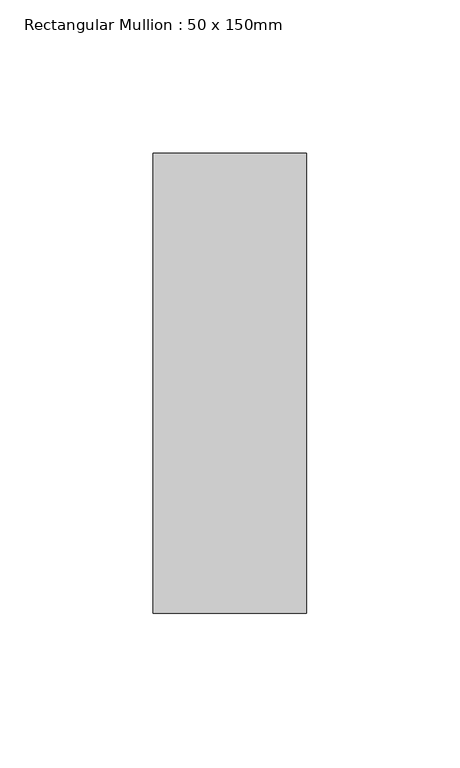
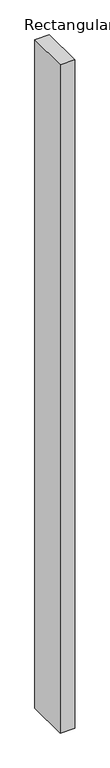
"""IFC4 building model written with IfcOpenShell, lengths in millimetres: member geometry, Rectangular Mullion : 50 x 150mm."""

from ifc_helpers import new_model, si_unit, frame, origin, place, context, project, spatial, polyline, outline, extrude, source, transform, mapped, element, save


def rectangular_mullion_50_x_150mm_fd5e96fe(model_context):
    return source(origin(), model_context, "Body", "SweptSolid", [
        extrude(outline(polyline([(0.0, 75.0), (0.0, -75.0), (-50.0, -75.0), (-50.0, 75.0), (0.0, 75.0)])), frame((0.0, 0.0, -2425.0), z_axis=(0.0, 0.0, 1.0), x_axis=(1.0, 0.0, 0.0)), (0.0, 0.0, 1.0), 2425.0),
    ])


if __name__ == "__main__":
    model = new_model("IFC4")
    model_context = context("Model", 3, world=origin())
    ifc_project = project(units=[si_unit("LENGTHUNIT", "METRE", prefix="MILLI")], contexts=[model_context])
    site = spatial("IfcSite", under=ifc_project)
    building = spatial("IfcBuilding", under=site)
    placement = place(None, origin())
    rectangular_mullion_50_x_150mm_shape = rectangular_mullion_50_x_150mm_fd5e96fe(model_context)
    element("IfcMember", 1, ObjectType="Rectangular Mullion : 50 x 150mm", at=placement, inside=building, context=model_context, shape_type="MappedRepresentation", body=[
        mapped(rectangular_mullion_50_x_150mm_shape, transform((0.0, 0.0, 0.0), x_axis=(1.0, 0.0, 0.0), y_axis=(0.0, 1.0, 0.0), z_axis=(0.0, 0.0, 1.0))),
    ])
    save(model, "model.ifc")

# Revit data of these elements
# Type "Rectangular Mullion : 50 x 150mm"
#   built-in parameter 1007304 = 0.492126 (stored number, unit not read)
#   built-in parameter 1007301 = 0.082021 (stored number, unit not read)
#   built-in parameter 1007300 = 0.082021 (stored number, unit not read)
# Element 1 (IfcMember, "Rectangular Mullion : 50 x 150mm")
#   Materials on its faces: "Aluminium"
# Materials
#   "Aluminium": class "Metal", colour RGB 247 247 247, transparency 0, Description = "Aluminium 6061", Cost = 0
